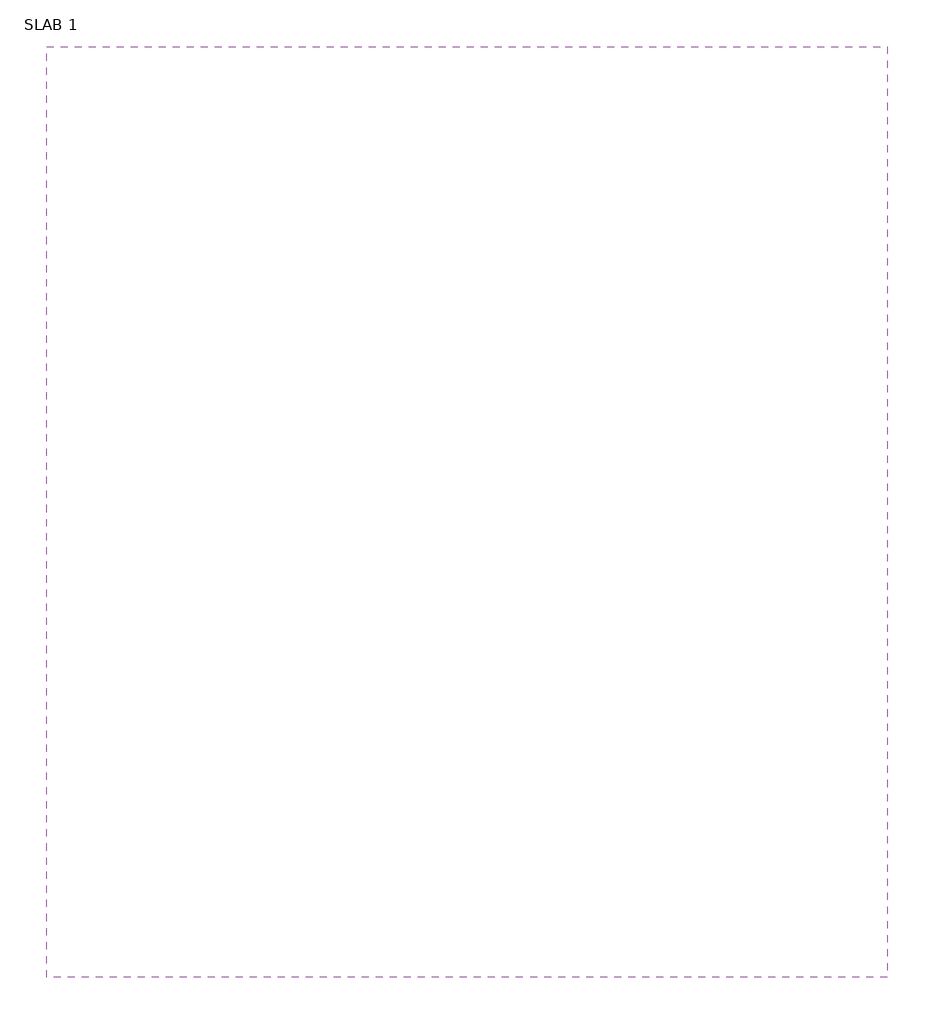
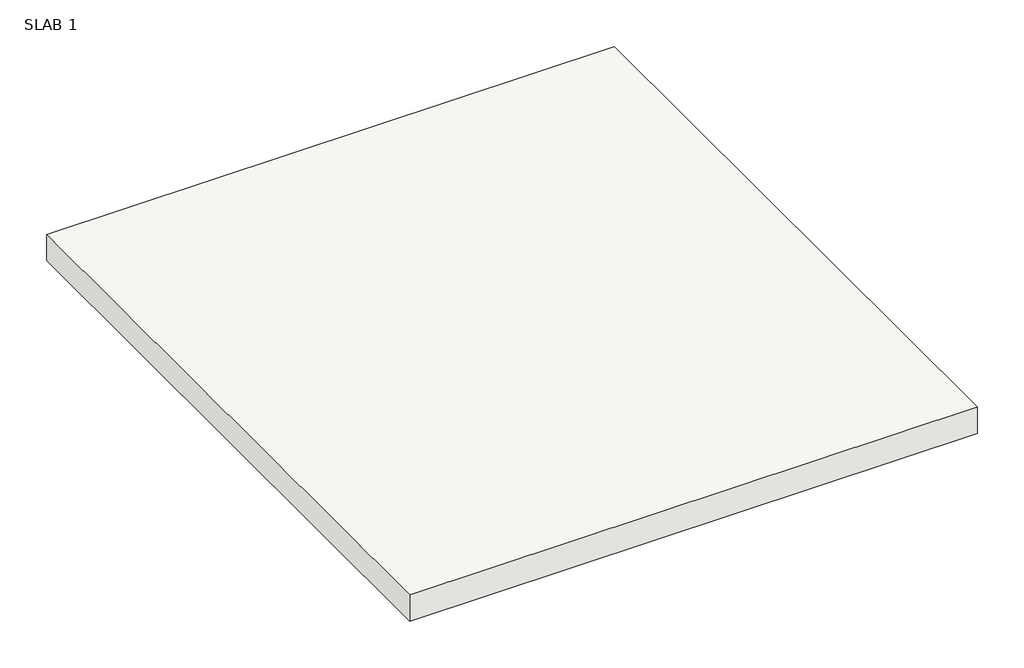
# One storey: 1 slab.
"""IFC4 building model written with IfcOpenShell, lengths in millimetres."""

from ifc_helpers import new_model, si_unit, frame, origin, place, context, project, spatial, polyline, outline, extrude, element, save

model = new_model("IFC4")

# Units and contexts
model_context = context("Model", 3, world=origin())
ifc_project = project(units=[si_unit("LENGTHUNIT", "METRE", prefix="MILLI")], contexts=[model_context])

# Site, building, storey
site = spatial("IfcSite", under=ifc_project)
building = spatial("IfcBuilding", under=site)
storey = spatial("IfcBuildingStorey", under=building, Name="SLAB 1", Elevation=3657.6)

# Slab
placement = place(None, origin())
element("IfcSlab", 1, ObjectType="Generic - 12\"", at=placement, inside=storey, context=model_context, shape_type="SweptSolid", body=[
    extrude(outline(polyline([(-743.3008651, 13448.6047421), (-743.3008651, -303.1418232), (-13163.9008651, -303.1418232), (-13163.9008651, 13448.6047421), (-743.3008651, 13448.6047421)])), frame((0.0, 0.0, 6400.8), z_axis=(0.0, 0.0, 1.0), x_axis=(1.0, 0.0, 0.0)), (0.0, 0.0, 1.0), 609.6),
])

save(model, "model.ifc")

# Revit data of these elements
# Type "Generic - 12\""
#   Assembly Code = "B1010"
#   Function = 0
#   Layers, outside or top first: 2' - 0" "Gypsum Wall Board" (function 1)
# Element 1 (IfcSlab, "Generic - 12\"")
#   Height Offset From Level = 11' - 0"
#   Phase Created = New Construction
#   Materials on its faces: "Gypsum Wall Board"
# Materials
#   "Gypsum Wall Board": class "Generic", colour RGB 127 127 127, transparency 0, Description = "Gypsum Wall Board", Cost = 0
